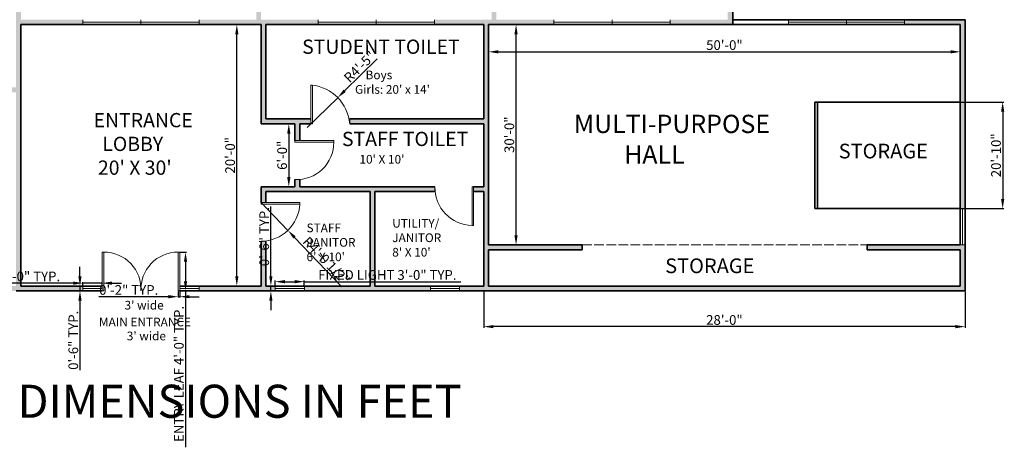
# Model space of a CAD drawing. Units: inches. Extents: x 2623 to 5095, y 1050 to 2384.
# Tile 3 of 4: x 3768 to 4988, y 1050 to 1580. Entities that reach past the tile are written whole.
import ezdxf

# ---------------------------------------------------------------- set-up
doc = ezdxf.new("R2010")
doc.units = ezdxf.units.IN
doc.linetypes.add('ACAD_ISO02W100', pattern=[15, 12, -3])
for name, color, linetype, lineweight in [('A-ANNO-DIMS', 2, 'Continuous', 13), ('A-ANNO-TEXT', 7, 'Continuous', 18), ('A-ANNO-TITL', 7, 'Continuous', 25), ('A-AREA-IDEN', 7, 'Continuous', 18), ('A-DOOR', 3, 'Continuous', 18), ('A-GLAZ', 4, 'Continuous', 18), ('A-WALL', 7, 'Continuous', 35), ('A-WALL-OVHD', 7, 'ACAD_ISO02W100', 18)]:
    doc.layers.add(name, color=color, linetype=linetype, lineweight=lineweight)
doc.layers.add('A-WALL-PATT', color=251, linetype='Continuous', lineweight=9, true_color=0x636466)
doc.styles.get("Standard").update_dxf_attribs({"font": 'arial.ttf'})
doc.dimstyles.new('ISO-25', dxfattribs={"dimtxt": 12, "dimasz": 12, "dimexe": 1.25, "dimexo": 0.625, "dimtad": 1, "dimlunit": 3, "dimtxsty": 'Standard', "dimcen": 2.5, "dimadec": 0, "dimazin": 0, "dimtfac": 1, "dimtmove": 0, "dimatfit": 3, "dimfxl": 1, "dimarcsym": 0})

# ---------------------------------------------------------------- blocks, each defined once
blk = doc.blocks.new('*D16')
at = {"layer": 'A-ANNO-DIMS', "color": 0, "lineweight": -2, "transparency": 16777216}
for p, q in [((4343.3, 1243), (4343.3, 1198)), ((4939.7, 1243), (4939.7, 1198)), ((4927.7, 1199.3), (4355.3, 1199.3))]:
    blk.add_line(p, q, dxfattribs=at)
at = {"layer": 'A-ANNO-DIMS', "color": 0, "transparency": 16777216}
for points in [[(4355.3, 1201.3), (4355.3, 1197.3), (4343.3, 1199.3)], [(4927.7, 1201.3), (4927.7, 1197.3), (4939.7, 1199.3)]]:
    blk.add_solid(points, dxfattribs=at)
at = {"layer": 'Defpoints', "color": 0, "transparency": 16777216}
for p in [(4343.3, 1243.6), (4939.7, 1243.6), (4343.3, 1199.3)]:
    blk.add_point(p, dxfattribs=at)
at = {"layer": 'A-ANNO-DIMS', "color": 0, "transparency": 16777216, "insert": (4641.5, 1206), "char_height": 12, "attachment_point": 5}
blk.add_mtext('28\'-0"', dxfattribs=at)
blk = doc.blocks.new('*D17')
at = {"layer": 'A-ANNO-DIMS', "color": 0, "lineweight": -2, "transparency": 16777216}
for p, q in [((4934.3, 1477.6), (4987.6, 1477.6)), ((4986.3, 1465.6), (4986.3, 1357.6)), ((4934.3, 1345.6), (4987.6, 1345.6))]:
    blk.add_line(p, q, dxfattribs=at)
at = {"layer": 'A-ANNO-DIMS', "color": 0, "transparency": 16777216}
for points in [[(4984.3, 1465.6), (4988.3, 1465.6), (4986.3, 1477.6)], [(4984.3, 1357.6), (4988.3, 1357.6), (4986.3, 1345.6)]]:
    blk.add_solid(points, dxfattribs=at)
at = {"layer": 'Defpoints', "color": 0, "transparency": 16777216}
for p in [(4933.7, 1477.6), (4933.7, 1345.6), (4986.3, 1345.6)]:
    blk.add_point(p, dxfattribs=at)
at = {"layer": 'A-ANNO-DIMS', "color": 0, "transparency": 16777216, "insert": (4979.6, 1411.6), "char_height": 12, "attachment_point": 5, "rotation": 90}
blk.add_mtext('20\'-10"', dxfattribs=at)
blk = doc.blocks.new('*D27')
at = {"layer": 'A-ANNO-DIMS', "color": 0, "lineweight": -2, "transparency": 16777216}
for p, q in [((4066.7, 1573.6), (4036, 1573.6)), ((4037.3, 1261.6), (4037.3, 1561.6)), ((4066.7, 1249.6), (4036, 1249.6))]:
    blk.add_line(p, q, dxfattribs=at)
at = {"layer": 'A-ANNO-DIMS', "color": 0, "transparency": 16777216}
for points in [[(4035.3, 1561.6), (4039.3, 1561.6), (4037.3, 1573.6)], [(4035.3, 1261.6), (4039.3, 1261.6), (4037.3, 1249.6)]]:
    blk.add_solid(points, dxfattribs=at)
at = {"layer": 'Defpoints', "color": 0, "transparency": 16777216}
for p in [(4037.3, 1573.6), (4067.3, 1573.6), (4067.3, 1249.6)]:
    blk.add_point(p, dxfattribs=at)
at = {"layer": 'A-ANNO-DIMS', "color": 0, "transparency": 16777216, "insert": (4030.5, 1411.6), "char_height": 12, "attachment_point": 5, "rotation": 90}
blk.add_mtext('20\'-0"', dxfattribs=at)
blk = doc.blocks.new('*D28')
at = {"layer": 'A-ANNO-DIMS', "color": 0, "lineweight": -2, "transparency": 16777216}
for p, q in [((4108.7, 1450.6), (4100.5, 1450.6)), ((4101.7, 1438.6), (4101.7, 1384.6)), ((4108.7, 1372.6), (4100.5, 1372.6))]:
    blk.add_line(p, q, dxfattribs=at)
at = {"layer": 'A-ANNO-DIMS', "color": 0, "transparency": 16777216}
for points in [[(4099.7, 1438.6), (4103.7, 1438.6), (4101.7, 1450.6)], [(4099.7, 1384.6), (4103.7, 1384.6), (4101.7, 1372.6)]]:
    blk.add_solid(points, dxfattribs=at)
at = {"layer": 'Defpoints', "color": 0, "transparency": 16777216}
for p in [(4109.3, 1450.6), (4101.7, 1372.6), (4109.3, 1372.6)]:
    blk.add_point(p, dxfattribs=at)
at = {"layer": 'A-ANNO-DIMS', "color": 0, "transparency": 16777216, "insert": (4095, 1411.6), "char_height": 12, "attachment_point": 5, "rotation": 90}
blk.add_mtext('6\'-0"', dxfattribs=at)
blk = doc.blocks.new('*D29')
at = {"layer": 'A-ANNO-DIMS', "color": 0, "lineweight": -2, "transparency": 16777216}
for p, q in [((4349.9, 1573.6), (4384.5, 1573.6)), ((4383.3, 1312.6), (4383.3, 1561.6)), ((4349.9, 1300.6), (4384.5, 1300.6))]:
    blk.add_line(p, q, dxfattribs=at)
at = {"layer": 'A-ANNO-DIMS', "color": 0, "transparency": 16777216}
for points in [[(4381.3, 1561.6), (4385.3, 1561.6), (4383.3, 1573.6)], [(4381.3, 1312.6), (4385.3, 1312.6), (4383.3, 1300.6)]]:
    blk.add_solid(points, dxfattribs=at)
at = {"layer": 'Defpoints', "color": 0, "transparency": 16777216}
for p in [(4349.3, 1573.6), (4383.3, 1573.6), (4349.3, 1300.6)]:
    blk.add_point(p, dxfattribs=at)
at = {"layer": 'A-ANNO-DIMS', "color": 0, "transparency": 16777216, "insert": (4376.5, 1437.1), "char_height": 12, "attachment_point": 5, "rotation": 90}
blk.add_mtext('30\'-0"', dxfattribs=at)
blk = doc.blocks.new('*D30')
at = {"layer": 'A-ANNO-DIMS', "color": 0, "lineweight": -2, "transparency": 16777216}
for p, q in [((4349.3, 1573), (4349.3, 1538.6)), ((4933.7, 1573), (4933.7, 1538.6)), ((4361.3, 1539.8), (4921.7, 1539.8))]:
    blk.add_line(p, q, dxfattribs=at)
at = {"layer": 'A-ANNO-DIMS', "color": 0, "transparency": 16777216}
for points in [[(4361.3, 1541.8), (4361.3, 1537.8), (4349.3, 1539.8)], [(4921.7, 1541.8), (4921.7, 1537.8), (4933.7, 1539.8)]]:
    blk.add_solid(points, dxfattribs=at)
at = {"layer": 'Defpoints', "color": 0, "transparency": 16777216}
for p in [(4349.3, 1573.6), (4933.7, 1573.6), (4933.7, 1539.8)]:
    blk.add_point(p, dxfattribs=at)
at = {"layer": 'A-ANNO-DIMS', "color": 0, "transparency": 16777216, "insert": (4641.5, 1546.6), "char_height": 12, "attachment_point": 5}
blk.add_mtext('50\'-0"', dxfattribs=at)
blk = doc.blocks.new('WIN-144-DOUBLE-LIGHT')
for p, q in [((0, 6), (0, 0)), ((144, 3), (0, 3)), ((72, 6), (72, 0)), ((144, 6), (144, 0))]:
    blk.add_line(p, q)
blk = doc.blocks.new('WIN-36-FIXED')
for p, q in [((0, 6), (0, 0)), ((0, 3), (36, 3)), ((36, 6), (36, 0))]:
    blk.add_line(p, q)
blk = doc.blocks.new('SIDELIGHT-24')
for p, q in [((0, 6), (0, 0)), ((0, 3), (24, 3)), ((24, 0), (24, 6))]:
    blk.add_line(p, q)
blk = doc.blocks.new('DOOR-48-LEAF-AND-JAMBS')
for p, q in [((0, 48), (0, 0)), ((2, 48), (0, 48)), ((0, 48), (0, 42)), ((2, 0), (2, 48)), ((48, 48), (48, 42)), ((0, 0), (2, 0))]:
    blk.add_line(p, q)
blk = doc.blocks.new('DOOR-48-ENTRY-LEAF')
for p, q in [((0, 0), (0, 48)), ((0, 48), (2, 48)), ((2, 48), (2, 0)), ((2, 0), (0, 0))]:
    blk.add_line(p, q)
blk = doc.blocks.new('*D59')
at = {"layer": 'A-ANNO-DIMS', "color": 0, "lineweight": -2, "transparency": 16777216}
for p, q in [((4084.9, 1250.2), (4084.9, 1256.3)), ((4096.9, 1255), (4108.9, 1255)), ((4120.9, 1250.2), (4120.9, 1256.3)), ((4120.9, 1255), (4314.7, 1255))]:
    blk.add_line(p, q, dxfattribs=at)
at = {"layer": 'A-ANNO-DIMS', "color": 0, "transparency": 16777216}
for points in [[(4096.9, 1257), (4096.9, 1253), (4084.9, 1255)], [(4108.9, 1257), (4108.9, 1253), (4120.9, 1255)]]:
    blk.add_solid(points, dxfattribs=at)
at = {"layer": 'Defpoints', "color": 0, "transparency": 16777216}
for p in [(4084.9, 1249.6), (4120.9, 1255), (4120.9, 1249.6)]:
    blk.add_point(p, dxfattribs=at)
at = {"layer": 'A-ANNO-DIMS', "color": 0, "transparency": 16777216, "insert": (4223.8, 1261.8), "char_height": 12, "attachment_point": 5}
blk.add_mtext('FIXED LIGHT 3\'-0" TYP.', dxfattribs=at)
blk = doc.blocks.new('*D60')
at = {"layer": 'A-ANNO-DIMS', "color": 0, "lineweight": -2, "transparency": 16777216}
for p, q in [((4079.5, 1261.6), (4079.5, 1348)), ((4084.3, 1249.6), (4078.3, 1249.6)), ((4079.5, 1243.6), (4079.5, 1249.6)), ((4084.3, 1243.6), (4078.3, 1243.6)), ((4079.5, 1231.6), (4079.5, 1219.6))]:
    blk.add_line(p, q, dxfattribs=at)
at = {"layer": 'A-ANNO-DIMS', "color": 0, "transparency": 16777216}
for points in [[(4077.5, 1261.6), (4081.5, 1261.6), (4079.5, 1249.6)], [(4077.5, 1231.6), (4081.5, 1231.6), (4079.5, 1243.6)]]:
    blk.add_solid(points, dxfattribs=at)
at = {"layer": 'Defpoints', "color": 0, "transparency": 16777216}
for p in [(4079.5, 1249.6), (4084.9, 1249.6), (4084.9, 1243.6)]:
    blk.add_point(p, dxfattribs=at)
at = {"layer": 'A-ANNO-DIMS', "color": 0, "transparency": 16777216, "insert": (4072.8, 1310.8), "char_height": 12, "attachment_point": 5, "rotation": 90}
blk.add_mtext('0\'-6" TYP.', dxfattribs=at)
blk = doc.blocks.new('*D61')
at = {"layer": 'A-ANNO-DIMS', "color": 0, "lineweight": -2, "transparency": 16777216}
for p, q in [((3967.1, 1291.6), (3975, 1291.6)), ((3973.7, 1279.6), (3973.7, 1255.6)), ((3967.1, 1243.6), (3975, 1243.6)), ((3973.7, 1243.6), (3973.7, 1049.8))]:
    blk.add_line(p, q, dxfattribs=at)
at = {"layer": 'A-ANNO-DIMS', "color": 0, "transparency": 16777216}
for points in [[(3971.7, 1279.6), (3975.7, 1279.6), (3973.7, 1291.6)], [(3971.7, 1255.6), (3975.7, 1255.6), (3973.7, 1243.6)]]:
    blk.add_solid(points, dxfattribs=at)
at = {"layer": 'Defpoints', "color": 0, "transparency": 16777216}
for p in [(3966.5, 1291.6), (3966.5, 1243.6), (3973.7, 1243.6)]:
    blk.add_point(p, dxfattribs=at)
at = {"layer": 'A-ANNO-DIMS', "color": 0, "transparency": 16777216, "insert": (3967, 1140.7), "char_height": 12, "attachment_point": 5, "rotation": 90}
blk.add_mtext('ENTRY LEAF 4\'-0" TYP.', dxfattribs=at)
blk = doc.blocks.new('*D62')
at = {"layer": 'A-ANNO-DIMS', "color": 0, "lineweight": -2, "transparency": 16777216}
for p, q in [((3952.5, 1236.4), (3866.1, 1236.4)), ((3964.5, 1243), (3964.5, 1235.2)), ((3966.5, 1236.4), (3964.5, 1236.4)), ((3966.5, 1243), (3966.5, 1235.2)), ((3978.5, 1236.4), (3990.5, 1236.4))]:
    blk.add_line(p, q, dxfattribs=at)
at = {"layer": 'A-ANNO-DIMS', "color": 0, "transparency": 16777216}
for points in [[(3952.5, 1238.4), (3952.5, 1234.4), (3964.5, 1236.4)], [(3978.5, 1238.4), (3978.5, 1234.4), (3966.5, 1236.4)]]:
    blk.add_solid(points, dxfattribs=at)
at = {"layer": 'Defpoints', "color": 0, "transparency": 16777216}
for p in [(3964.5, 1243.6), (3964.5, 1236.4), (3966.5, 1243.6)]:
    blk.add_point(p, dxfattribs=at)
at = {"layer": 'A-ANNO-DIMS', "color": 0, "transparency": 16777216, "insert": (3903.3, 1243.2), "char_height": 12, "attachment_point": 5}
blk.add_mtext('0\'-2" TYP.', dxfattribs=at)
blk = doc.blocks.new('*D63')
at = {"layer": 'A-ANNO-DIMS', "color": 0, "lineweight": -2, "transparency": 16777216}
for p, q in [((3834.5, 1253.2), (3655, 1253.2)), ((3846.5, 1250.2), (3846.5, 1254.5)), ((3870.5, 1253.2), (3846.5, 1253.2)), ((3870.5, 1250.2), (3870.5, 1254.5)), ((3882.5, 1253.2), (3894.5, 1253.2))]:
    blk.add_line(p, q, dxfattribs=at)
at = {"layer": 'A-ANNO-DIMS', "color": 0, "transparency": 16777216}
for points in [[(3834.5, 1255.2), (3834.5, 1251.2), (3846.5, 1253.2)], [(3882.5, 1255.2), (3882.5, 1251.2), (3870.5, 1253.2)]]:
    blk.add_solid(points, dxfattribs=at)
at = {"layer": 'Defpoints', "color": 0, "transparency": 16777216}
for p in [(3846.5, 1253.2), (3846.5, 1249.6), (3870.5, 1249.6)]:
    blk.add_point(p, dxfattribs=at)
at = {"layer": 'A-ANNO-DIMS', "color": 0, "transparency": 16777216, "insert": (3738.8, 1260), "char_height": 12, "attachment_point": 5}
blk.add_mtext('SIDELIGHT 2\'-0" TYP.', dxfattribs=at)
blk = doc.blocks.new('*D64')
at = {"layer": 'A-ANNO-DIMS', "color": 0, "lineweight": -2, "transparency": 16777216}
for p, q in [((3842.9, 1261.6), (3842.9, 1273.6)), ((3845.9, 1249.6), (3841.7, 1249.6)), ((3842.9, 1249.6), (3842.9, 1243.6)), ((3845.9, 1243.6), (3841.7, 1243.6)), ((3842.9, 1231.6), (3842.9, 1145.2))]:
    blk.add_line(p, q, dxfattribs=at)
at = {"layer": 'A-ANNO-DIMS', "color": 0, "transparency": 16777216}
for points in [[(3840.9, 1261.6), (3844.9, 1261.6), (3842.9, 1249.6)], [(3840.9, 1231.6), (3844.9, 1231.6), (3842.9, 1243.6)]]:
    blk.add_solid(points, dxfattribs=at)
at = {"layer": 'Defpoints', "color": 0, "transparency": 16777216}
for p in [(3846.5, 1249.6), (3842.9, 1243.6), (3846.5, 1243.6)]:
    blk.add_point(p, dxfattribs=at)
at = {"layer": 'A-ANNO-DIMS', "color": 0, "transparency": 16777216, "insert": (3836.2, 1182.4), "char_height": 12, "attachment_point": 5, "rotation": 90}
blk.add_mtext('0\'-6" TYP.', dxfattribs=at)
blk = doc.blocks.new('*D68')
at = {"layer": 'A-ANNO-DIMS', "color": 0, "lineweight": -2, "transparency": 16777216}
for p, q in [((4211.3, 1531), (4170.8, 1491.4)), ((4124.4, 1446), (4162.3, 1483))]:
    blk.add_line(p, q, dxfattribs=at)
at = {"layer": 'A-ANNO-DIMS', "color": 0, "transparency": 16777216}
blk.add_solid([(4169.4, 1492.8), (4172.2, 1490), (4162.3, 1483)], dxfattribs=at)
at = {"layer": 'Defpoints', "color": 0, "transparency": 16777216}
for p in [(4162.3, 1483), (4124.4, 1446)]:
    blk.add_point(p, dxfattribs=at)
at = {"layer": 'A-ANNO-DIMS', "color": 0, "transparency": 16777216, "insert": (4190.6, 1520.2), "char_height": 12, "attachment_point": 5, "rotation": 44.3968}
blk.add_mtext('R4\'-5"', dxfattribs=at)
blk = doc.blocks.new('*D69')
at = {"layer": 'A-ANNO-DIMS', "color": 0, "lineweight": -2, "transparency": 16777216}
for p, q in [((4067, 1353.5), (4100.5, 1318.6)), ((4167.3, 1248.8), (4108.8, 1309.9))]:
    blk.add_line(p, q, dxfattribs=at)
at = {"layer": 'A-ANNO-DIMS', "color": 0, "transparency": 16777216}
blk.add_solid([(4110.2, 1311.3), (4107.3, 1308.5), (4100.5, 1318.6)], dxfattribs=at)
at = {"layer": 'Defpoints', "color": 0, "transparency": 16777216}
for p in [(4067, 1353.5), (4100.5, 1318.6)]:
    blk.add_point(p, dxfattribs=at)
at = {"layer": 'A-ANNO-DIMS', "color": 0, "transparency": 16777216, "insert": (4147.1, 1279.8), "char_height": 12, "attachment_point": 5, "rotation": 313.7814}
blk.add_mtext('R4\'-0 1/2"', dxfattribs=at)

msp = doc.modelspace()

# ---------------------------------------------------------------- hatches: boundary and pattern name
at = {"layer": 'A-WALL-PATT'}
h = msp.add_hatch(color=256, dxfattribs=at)
h.dxf.hatch_style = 1
h.paths.add_polyline_path([(3103.717, 2251.615), (2755.717, 2251.615), (2755.717, 2173.615), (2761.717, 2173.615), (2761.717, 2245.615), (3097.717, 2245.615), (3097.717, 2015.688), (3100.811, 2015.688, -0.01561511), (3103.717, 2015.688)])
h.paths.add_polyline_path([(3103.717, 1967.688), (3097.717, 1967.688), (3097.717, 1957.615), (2761.717, 1957.615), (2761.717, 2029.615), (2755.717, 2029.615), (2755.717, 1915.615), (2761.717, 1915.615), (2761.717, 1951.615), (3097.717, 1951.615), (3097.717, 1943.747), (3103.717, 1943.747)])
h.paths.add_polyline_path([(3103.717, 1895.747, -0.01327118), (3101.235, 1895.747), (3097.717, 1895.747), (3097.717, 1735.615), (2761.717, 1735.615), (2761.717, 1771.615), (2755.717, 1771.615), (2755.717, 1693.615), (2761.717, 1693.615), (2761.717, 1729.615), (3097.717, 1729.615), (3097.717, 1721.81), (3103.717, 1721.81)])
h.paths.add_polyline_path([(2761.717, 1573.615), (2755.717, 1573.615), (2755.717, 1405.615), (2761.717, 1405.615)])
h.paths.add_polyline_path([(2761.717, 1285.615), (2755.717, 1285.615), (2755.717, 1243.615), (2857.717, 1243.615), (2857.717, 1249.615), (2761.717, 1249.615)])
h.paths.add_polyline_path([(3152.017, 1249.615), (3103.717, 1249.615), (3103.717, 1489.615), (3237.319, 1489.615, -0.03349431), (3237.344, 1495.615), (3103.717, 1495.615), (3103.717, 1507.046), (3097.717, 1507.046), (3097.717, 1249.615), (3001.717, 1249.615), (3001.717, 1243.615), (3103.717, 1243.615), (3152.017, 1243.615)])
h.paths.add_polyline_path([(3103.717, 1673.81, -0.01537929), (3100.853, 1673.81), (3097.717, 1673.81), (3097.717, 1555.046), (3101.163, 1555.046, -0.01366836), (3103.717, 1555.046)])
h.paths.add_polyline_path([(3302.317, 1249.615), (3302.317, 1297.615), (3385.117, 1297.615), (3385.117, 1303.615), (3302.317, 1303.615), (3302.317, 1489.615), (3503.954, 1489.615), (3503.954, 1492.911, -0.01449155), (3503.954, 1495.615), (3285.344, 1495.615), (3285.344, 1489.615), (3296.317, 1489.615), (3296.317, 1249.615), (3248.017, 1249.615), (3248.017, 1243.615), (3302.317, 1243.615)])
h.paths.add_polyline_path([(3569.917, 1489.615), (3579.094, 1489.615), (3579.094, 1495.615), (3551.954, 1495.615), (3551.954, 1489.615), (3563.917, 1489.615), (3563.917, 1303.615), (3481.117, 1303.615), (3481.117, 1297.615), (3563.917, 1297.615), (3563.917, 1249.615), (3563.917, 1243.615), (3618.817, 1243.615), (3618.817, 1249.615), (3569.917, 1249.615)])
h.paths.add_polyline_path([(3846.517, 1249.615), (3769.717, 1249.615), (3769.717, 1573.615), (3846.517, 1573.615), (3846.517, 1579.615), (3769.717, 1579.615), (3769.717, 1654.615), (3763.717, 1654.615), (3763.717, 1495.615), (3627.094, 1495.615, -0.01677945), (3627.094, 1492.499), (3627.094, 1489.615), (3763.717, 1489.615), (3763.717, 1249.615), (3714.817, 1249.615), (3714.817, 1243.615), (3763.717, 1243.615), (3846.517, 1243.615)])
h.paths.add_polyline_path([(4084.941, 1249.615), (4073.317, 1249.615), (4073.317, 1305.13), (4067.317, 1305.13), (4067.317, 1249.615), (3990.517, 1249.615), (3990.517, 1243.615), (4084.941, 1243.615)])
h.paths.add_polyline_path([(4277.411, 1249.615), (4208.317, 1249.615), (4208.317, 1366.615), (4282.724, 1366.615), (4282.724, 1370.675, -0.01031167), (4282.724, 1372.615), (4115.317, 1372.615), (4115.317, 1381.792), (4114.62, 1381.792, -0.02925374), (4109.317, 1381.792), (4109.317, 1372.615), (4073.317, 1372.615), (4067.317, 1372.615), (4067.317, 1353.13), (4073.317, 1353.13), (4073.317, 1366.615), (4202.317, 1366.615), (4202.317, 1249.615), (4120.941, 1249.615), (4120.941, 1243.615), (4277.411, 1243.615)])
h.paths.add_polyline_path([(4939.717, 1300.615), (4933.717, 1300.615), (4818.498, 1300.615), (4818.498, 1294.615), (4933.717, 1294.615), (4933.717, 1249.615), (4349.317, 1249.615), (4349.317, 1294.615), (4465.249, 1294.615), (4465.249, 1300.615), (4349.317, 1300.615), (4349.317, 1573.615), (4430.317, 1573.615), (4430.317, 1579.615), (4358.917, 1579.615), (4358.917, 1873.615), (4365.566, 1873.615), (4365.566, 1879.615), (4345.539, 1879.615), (4345.539, 1873.615), (4352.917, 1873.615), (4352.917, 1579.615), (4282.117, 1579.615), (4282.117, 1573.615), (4343.317, 1573.615), (4343.317, 1456.615), (4177.166, 1456.615), (4177.166, 1450.615), (4343.317, 1450.615), (4343.317, 1372.615), (4330.724, 1372.615), (4330.724, 1366.615), (4343.317, 1366.615), (4343.317, 1249.615), (4313.411, 1249.615), (4313.411, 1243.615), (4939.717, 1243.615)])
h = msp.add_hatch(color=256, dxfattribs=at)
h.dxf.hatch_style = 1
h.paths.add_polyline_path([(4651.717, 1615.615), (4975.717, 1615.615), (4975.717, 1657.615), (4969.717, 1657.615), (4969.717, 1621.615), (4729.717, 1621.615), (4729.717, 1741.615), (4735.396, 1741.615), (4735.396, 1747.615), (4723.717, 1747.615), (4723.717, 1621.615), (4651.717, 1621.615), (4651.717, 1654.615), (4645.717, 1654.615), (4645.717, 1579.615), (4574.317, 1579.615), (4574.317, 1573.615), (4651.717, 1573.615)])
h.paths.add_polyline_path([(4939.717, 1579.615), (4864.717, 1579.615), (4864.717, 1573.615), (4933.717, 1573.615), (4933.717, 1345.615), (4939.717, 1345.615)])
h.paths.add_polyline_path([(4975.717, 1804.615), (4969.717, 1804.615), (4969.717, 1747.615), (4783.396, 1747.615, -0.01744529), (4783.396, 1744.379), (4783.396, 1741.615), (4969.717, 1741.615), (4969.717, 1705.615), (4975.717, 1705.615)])
h.paths.add_polyline_path([(4975.717, 2047.615), (4969.717, 2047.615), (4969.717, 2011.615), (4785.608, 2011.615), (4785.608, 2008.9, -0.01771988), (4785.608, 2005.615), (4969.717, 2005.615), (4969.717, 1948.615), (4975.717, 1948.615), (4975.717, 2005.615)])
h.paths.add_polyline_path([(4975.717, 2137.615), (4729.717, 2137.615), (4723.717, 2137.615), (4723.717, 2005.615), (4737.608, 2005.615), (4737.608, 2011.615), (4729.717, 2011.615), (4729.717, 2131.615), (4969.717, 2131.615), (4969.717, 2095.615), (4975.717, 2095.615)])
h.paths.add_polyline_path([(4651.717, 2209.615), (4573.717, 2209.615), (4573.717, 2203.615), (4645.717, 2203.615), (4645.717, 2128.615), (4651.717, 2128.615)])
h.paths.add_polyline_path([(4651.717, 2032.615), (4645.717, 2032.615), (4645.717, 1957.615), (4413.911, 1957.615), (4413.911, 1956.398, -0.02623296), (4413.911, 1951.615), (4651.717, 1951.615)])
h.paths.add_polyline_path([(4357.717, 2203.615), (4429.717, 2203.615), (4429.717, 2209.615), (4279.717, 2209.615), (4279.717, 2203.615), (4351.717, 2203.615), (4351.717, 1957.615), (4345.154, 1957.615), (4345.154, 1951.615), (4365.911, 1951.615), (4365.911, 1957.615), (4357.717, 1957.615)])
h.paths.add_polyline_path([(4063.717, 2203.615), (4135.717, 2203.615), (4135.717, 2209.615), (3985.717, 2209.615), (3985.717, 2203.615), (4057.717, 2203.615), (4057.717, 1957.615), (3823.079, 1957.615), (3823.079, 1955.024, -0.01841239), (3823.079, 1951.615), (4075.656, 1951.615), (4075.656, 1957.615), (4063.717, 1957.615)])
h.paths.add_polyline_path([(4297.09, 1957.615), (4123.656, 1957.615), (4123.656, 1954.68, -0.01649439), (4123.656, 1951.615), (4297.154, 1951.615, -0.03370804)])
h.paths.add_polyline_path([(3769.717, 2203.615), (3841.717, 2203.615), (3841.717, 2209.615), (3691.717, 2209.615), (3691.717, 2203.615), (3763.717, 2203.615), (3763.717, 1957.615), (3754.594, 1957.615), (3754.594, 1951.615), (3775.079, 1951.615), (3775.079, 1957.615), (3769.717, 1957.615)])
h.paths.add_polyline_path([(3706.594, 1957.102), (3706.594, 1957.615), (3529.616, 1957.615), (3529.616, 1955.888, -0.02330465), (3529.616, 1951.615), (3706.594, 1951.615, -0.03033114)])
h.paths.add_polyline_path([(3481.616, 1957.615), (3475.717, 1957.615), (3475.717, 2203.615), (3547.717, 2203.615), (3547.717, 2209.615), (3397.717, 2209.615), (3397.717, 2203.615), (3469.717, 2203.615), (3469.717, 1957.615), (3457.307, 1957.615), (3457.307, 1951.615), (3481.616, 1951.615)])
h.paths.add_polyline_path([(3409.307, 1954.491), (3409.307, 1957.615), (3181.717, 1957.615), (3181.717, 2203.615), (3253.717, 2203.615), (3253.717, 2209.615), (3175.717, 2209.615), (3175.717, 1747.615, -0.01406848), (3178.344, 1747.615), (3181.717, 1747.615), (3181.717, 1873.615), (3434.065, 1873.615), (3434.065, 1877.049, -0.01373428), (3434.065, 1879.615), (3181.717, 1879.615), (3181.717, 1951.615), (3409.307, 1951.615, -0.01544691)])
h.paths.add_polyline_path([(4651.717, 1879.615), (4413.566, 1879.615, -0.01934194), (4413.566, 1876.041), (4413.566, 1873.615), (4645.717, 1873.615), (4645.717, 1798.615), (4651.717, 1798.615)])
h.paths.add_polyline_path([(4138.117, 1579.615), (4067.317, 1579.615), (4067.317, 1873.615), (4073.262, 1873.615), (4073.262, 1879.615), (4055.249, 1879.615), (4055.249, 1873.615), (4061.317, 1873.615), (4061.317, 1579.615), (3990.517, 1579.615), (3990.517, 1573.615), (4067.317, 1573.615), (4067.317, 1450.615), (4109.317, 1450.615), (4109.317, 1429.792), (4115.317, 1429.792), (4115.317, 1450.615), (4129.166, 1450.615), (4129.166, 1456.615), (4073.317, 1456.615), (4073.317, 1573.615), (4138.117, 1573.615)])
h.paths.add_polyline_path([(4297.539, 1879.615), (4121.262, 1879.615, -0.02641892), (4121.262, 1874.8), (4121.262, 1873.615), (4297.539, 1873.615), (4297.539, 1876.326, -0.01774472)])
h.paths.add_polyline_path([(4007.249, 1879.615), (3763.717, 1879.615), (3763.717, 1798.615), (3769.717, 1798.615), (3769.717, 1873.615), (4007.249, 1873.615), (4007.249, 1876.064, -0.01921077)])
h.paths.add_polyline_path([(3715.717, 1573.615), (3469.717, 1573.615), (3469.717, 1567.615), (3715.717, 1567.615)])
h.paths.add_polyline_path([(3421.717, 1570.87), (3421.717, 1573.615), (3181.717, 1573.615), (3181.717, 1699.615), (3175.717, 1699.615), (3175.717, 1567.615), (3421.717, 1567.615, -0.01755055)])
h.paths.add_polyline_path([(3715.717, 1879.615), (3482.065, 1879.615), (3482.065, 1873.615), (3715.717, 1873.615)])

# ---------------------------------------------------------------- linework, layer by layer
at = {"layer": 'A-DOOR'}
msp.add_line((3918.517, 1249.615), (3918.517, 1243.615), dxfattribs=at)
for centre, radius, start, end in [((4124.431, 1445.989), 52.937, 5.013021, 83.780796), ((4111.969, 1427.069), 45.354, 266.648724, 0.913525), ((4329.756, 1371.645), 47.041, 178.818411, 268.743838), ((4067.002, 1353.502), 48.373, 270.373098, 357.189152), ((3872.78, 1245.825), 45.791, 357.233414, 90.328835), ((3964.279, 1245.802), 45.814, 89.701854, 182.735896)]:
    msp.add_arc(centre, radius, start, end, dxfattribs=at)
at = {"layer": 'A-GLAZ'}
for p, q in [((4933.717, 1345.615), (4939.717, 1345.615)), ((4936.717, 1345.615), (4936.717, 1300.615)), ((4933.717, 1300.615), (4939.717, 1300.615))]:
    msp.add_line(p, q, dxfattribs=at)
at = {"layer": 'A-WALL'}
for p, q in [((4651.717, 1615.615), (4651.717, 1573.615)), ((4651.717, 1579.615), (4939.717, 1579.615)), ((4939.717, 1579.615), (4939.717, 1243.615)), ((3769.717, 1573.615), (4067.317, 1573.615)), ((3769.717, 1573.615), (3769.717, 1249.615)), ((4067.317, 1573.615), (4067.317, 1450.615)), ((4073.317, 1573.615), (4073.317, 1456.615)), ((4073.317, 1573.615), (4343.317, 1573.615)), ((4343.317, 1573.615), (4343.317, 1456.615)), ((4349.317, 1573.615), (4349.317, 1300.615)), ((4349.317, 1573.615), (4651.717, 1573.615)), ((4651.717, 1573.615), (4933.717, 1573.615)), ((4933.717, 1573.615), (4933.717, 1300.615)), ((4753.717, 1477.615), (4753.717, 1345.615)), ((4753.717, 1477.615), (4756.717, 1477.615)), ((4756.717, 1477.615), (4756.717, 1345.615)), ((4756.717, 1477.615), (4933.717, 1477.615)), ((4073.317, 1456.615), (4129.166, 1456.615)), ((4177.166, 1456.615), (4343.317, 1456.615)), ((4067.317, 1450.615), (4109.317, 1450.615)), ((4109.317, 1450.615), (4109.317, 1429.792)), ((4115.317, 1450.615), (4115.317, 1429.792)), ((4115.317, 1450.615), (4129.166, 1450.615)), ((4177.166, 1450.615), (4343.317, 1450.615)), ((4343.317, 1450.615), (4343.317, 1372.615)), ((4109.317, 1381.792), (4109.317, 1372.615)), ((4115.317, 1381.792), (4115.317, 1372.615)), ((4073.317, 1372.615), (4067.317, 1372.615)), ((4067.317, 1372.615), (4067.317, 1353.13)), ((4073.317, 1372.615), (4109.317, 1372.615)), ((4073.317, 1366.615), (4202.317, 1366.615)), ((4073.317, 1366.615), (4073.317, 1353.13)), ((4115.317, 1372.615), (4282.724, 1372.615)), ((4202.317, 1366.615), (4202.317, 1249.615)), ((4208.317, 1366.615), (4208.317, 1249.615)), ((4208.317, 1366.615), (4282.724, 1366.615)), ((4330.724, 1372.615), (4343.317, 1372.615)), ((4330.724, 1366.615), (4343.317, 1366.615)), ((4343.317, 1366.615), (4343.317, 1249.615)), ((4753.717, 1345.615), (4756.717, 1345.615)), ((4756.717, 1345.615), (4933.717, 1345.615)), ((4067.317, 1305.13), (4067.317, 1249.615)), ((4073.317, 1305.13), (4073.317, 1249.615)), ((4349.317, 1300.615), (4465.249, 1300.615)), ((4349.317, 1294.615), (4465.249, 1294.615)), ((4349.317, 1294.615), (4349.317, 1249.615)), ((4465.249, 1300.615), (4465.249, 1294.615)), ((4818.498, 1300.615), (4818.498, 1294.615)), ((4818.498, 1300.615), (4933.717, 1300.615)), ((4818.498, 1294.615), (4933.717, 1294.615)), ((4933.717, 1294.615), (4933.717, 1249.615)), ((3769.717, 1249.615), (3870.517, 1249.615)), ((3966.517, 1249.615), (4067.317, 1249.615)), ((4073.317, 1249.615), (4202.317, 1249.615)), ((4208.317, 1249.615), (4343.317, 1249.615)), ((4349.317, 1249.615), (4933.717, 1249.615)), ((3763.717, 1243.615), (3870.517, 1243.615)), ((3966.517, 1243.615), (4939.717, 1243.615))]:
    msp.add_line(p, q, dxfattribs=at)
at = {"layer": 'A-WALL-OVHD'}
msp.add_line((4465.249, 1300.615), (4818.498, 1300.615), dxfattribs=at)

# ---------------------------------------------------------------- block references
at = {"layer": 'A-DOOR', "extrusion": (0, 0, -1), "zscale": -1}
for p, rotation in [((-4129.166, 1498.615), 180), ((-4157.317, 1429.792), 270.0000000000055), ((-4115.317, 1353.13), 270.0000000000057)]:
    msp.add_blockref('DOOR-48-LEAF-AND-JAMBS', p, dxfattribs=dict(at, rotation=rotation))
msp.add_blockref('DOOR-48-LEAF-AND-JAMBS', (-4330.724, 1324.615), dxfattribs=at)
at = {"layer": 'A-DOOR'}
msp.add_blockref('DOOR-48-ENTRY-LEAF', (3870.517, 1243.615), dxfattribs=at)
at = {"layer": 'A-DOOR', "rotation": 180}
msp.add_blockref('DOOR-48-ENTRY-LEAF', (3966.517, 1291.615), dxfattribs=at)
at = {"layer": 'A-GLAZ'}
for name, p in [('WIN-144-DOUBLE-LIGHT', (3846.517, 1573.615)), ('WIN-144-DOUBLE-LIGHT', (4138.117, 1573.615)), ('WIN-144-DOUBLE-LIGHT', (4430.317, 1573.615)), ('SIDELIGHT-24', (3966.517, 1243.615)), ('WIN-36-FIXED', (4084.941, 1243.615)), ('WIN-36-FIXED', (4277.411, 1243.615))]:
    msp.add_blockref(name, p, dxfattribs=at)
at = {"layer": 'A-GLAZ', "rotation": 180}
for name, p in [('WIN-144-DOUBLE-LIGHT', (4864.717, 1579.615)), ('SIDELIGHT-24', (3870.517, 1249.615))]:
    msp.add_blockref(name, p, dxfattribs=at)

# ---------------------------------------------------------------- texts
at = {"layer": 'A-ANNO-TEXT', "attachment_point": 1}
for s, insert, char_height in [("3' wide", (3898.131, 1231.225), 10.7617), ('MAIN ENTRANCE', (3866.439, 1210.383), 10.76174), ("3' wide", (3900.936, 1193.128), 10.7617)]:
    msp.add_mtext_dynamic_manual_height_columns(s, width=391.78395, gutter_width=53.809, heights=[0], dxfattribs=dict(at, insert=insert, char_height=char_height))
at = {"layer": 'A-ANNO-TITL', "insert": (2779.618, 1127.325), "char_height": 40.95464, "attachment_point": 1}
msp.add_mtext_dynamic_manual_height_columns('MODERN PRIMARY SCHOOL PLAN ALL DIMENSIONS IN FEET', width=1853.61769, gutter_width=204.773, heights=[0], dxfattribs=at)
at = {"layer": 'A-AREA-IDEN', "attachment_point": 1}
for s, width, gutter_width, insert, char_height in [('STUDENT TOILET', 642.72757, 88.274, (4118.233, 1554.954), 17.6548), ("    Boys \\PGirls: 20' x 14'", 391.78395, 53.809, (4183.695, 1516.563), 10.76174), ("ENTRANCE\\P  LOBBY\\P 20' X 30'", 642.72757, 88.274, (3859.796, 1463.994), 17.6548), ('MULTI-PURPOSE \\P         HALL', 824.72693, 113.27, (4454.973, 1461.819), 22.65406), ('STAFF TOILET', 642.72757, 88.274, (4167.579, 1440.677), 17.6548), ('STORAGE', 661.86265, 90.902, (4783.105, 1425.926), 18.1804), ("10' X 10'", 391.78395, 53.809, (4189.231, 1412.03), 10.7617), ("UTILITY/\\PJANITOR\\P8' X 10'", 391.78395, 53.809, (4229.864, 1332.771), 10.7617), ("STAFF\\PJANITOR\\P6' X 10'", 391.78395, 53.809, (4123.648, 1327.025), 10.7617), ('STORAGE', 661.86265, 90.902, (4568.089, 1283.784), 18.1804)]:
    msp.add_mtext_dynamic_manual_height_columns(s, width=width, gutter_width=gutter_width, heights=[0], dxfattribs=dict(at, insert=insert, char_height=char_height))

# ---------------------------------------------------------------- dimensions: what is measured, and where the dimension line sits
at = {"layer": 'A-ANNO-DIMS'}
for base, p1, p2, angle, text, override, picture, middle in [((4037.289, 1573.615), (4067.317, 1249.615), (4067.317, 1573.615), 90, '20\'-0"', {"dimclrd": 0, "dimclre": 0, "dimclrt": 0}, '*D27', (4030.537, 1411.615)), ((4383.26, 1573.615), (4349.317, 1300.615), (4349.317, 1573.615), 90, '30\'-0"', {"dimclrd": 0, "dimclre": 0, "dimclrt": 0}, '*D29', (4376.504, 1437.115)), ((4986.326, 1345.615), (4933.717, 1477.615), (4933.717, 1345.615), 90, '20\'-10"', {"dimclrd": 0, "dimclre": 0, "dimclrt": 0}, '*D17', (4979.574, 1411.615)), ((4101.705, 1372.615), (4109.317, 1450.615), (4109.317, 1372.615), 90, '6\'-0"', {"dimclrd": 0, "dimclre": 0, "dimclrt": 0}, '*D28', (4094.953, 1411.615)), ((4079.541, 1249.615), (4084.941, 1243.615), (4084.941, 1249.615), 90, '<> TYP.', {"dimdec": 1, "dimlfac": 1, "dimrnd": 0, "dimzin": 1, "dimdsep": 46, "dimlunit": 4, "dimfrac": 2}, '*D60', (4072.789, 1310.813)), ((3846.517, 1253.215), (3870.517, 1249.615), (3846.517, 1249.615), 180, 'SIDELIGHT <> TYP.', {"dimdec": 1, "dimlfac": 1, "dimrnd": 0, "dimzin": 1, "dimdsep": 46, "dimlunit": 4, "dimfrac": 2}, '*D63', (3738.772, 1260.045)), ((3973.717, 1243.615), (3966.517, 1291.615), (3966.517, 1243.615), 270, 'ENTRY LEAF <> TYP.', {"dimdec": 1, "dimlfac": 1, "dimrnd": 0, "dimzin": 1, "dimdsep": 46, "dimlunit": 4, "dimfrac": 2}, '*D61', (3966.966, 1140.703)), ((3842.917, 1243.615), (3846.517, 1249.615), (3846.517, 1243.615), 270, '<> TYP.', {"dimdec": 1, "dimlfac": 1, "dimrnd": 0, "dimzin": 1, "dimdsep": 46, "dimlunit": 4, "dimfrac": 2}, '*D64', (3836.166, 1182.417)), ((3964.517, 1236.415), (3966.517, 1243.615), (3964.517, 1243.615), 180, '<> TYP.', {"dimdec": 1, "dimlfac": 1, "dimrnd": 0, "dimzin": 1, "dimdsep": 46, "dimlunit": 4, "dimfrac": 2}, '*D62', (3903.319, 1243.167))]:
    dim = msp.add_linear_dim(base=base, p1=p1, p2=p2, angle=angle, text=text, dimstyle='ISO-25', override=override, dxfattribs=at)
    dim.commit()
    dim.dimension.update_dxf_attribs({"geometry": picture, "text_midpoint": middle})
for base, p1, p2, text, override, picture, middle in [((4933.717, 1539.803), (4349.317, 1573.615), (4933.717, 1573.615), '50\'-0"', {"dimclrd": 0, "dimclre": 0, "dimclrt": 0}, '*D30', (4641.517, 1546.555)), ((4120.941, 1255.015), (4084.941, 1249.615), (4120.941, 1249.615), 'FIXED LIGHT <> TYP.', {"dimdec": 1, "dimlfac": 1, "dimrnd": 0, "dimzin": 1, "dimdsep": 46, "dimlunit": 4, "dimfrac": 2}, '*D59', (4223.823, 1261.849)), ((4343.317, 1199.262), (4939.717, 1243.615), (4343.317, 1243.615), '28\'-0"', {"dimclrd": 0, "dimclre": 0, "dimclrt": 0}, '*D16', (4641.517, 1206.014))]:
    dim = msp.add_linear_dim(base=base, p1=p1, p2=p2, text=text, dimstyle='ISO-25', override=override, dxfattribs=at)
    dim.commit()
    dim.dimension.update_dxf_attribs({"geometry": picture, "text_midpoint": middle})
for center, mpoint, picture, middle in [((4124.431, 1445.989), (4162.255, 1483.025), '*D68', (4190.643, 1520.236)), ((4067.002, 1353.502), (4100.472, 1318.578), '*D69', (4147.124, 1279.769))]:
    dim = msp.add_radius_dim(center=center, mpoint=mpoint, dimstyle='ISO-25', override={"dimdec": 1, "dimlfac": 1, "dimrnd": 0, "dimzin": 1, "dimdsep": 46, "dimlunit": 4, "dimfrac": 2}, dxfattribs=at)
    dim.commit()
    dim.dimension.update_dxf_attribs({"geometry": picture, "text_midpoint": middle})

doc.saveas('drawing.dxf')
